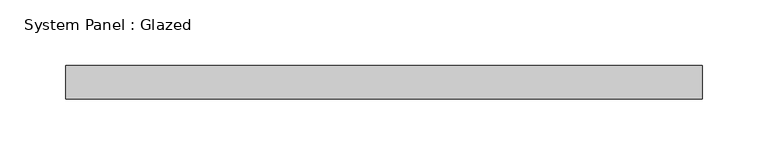
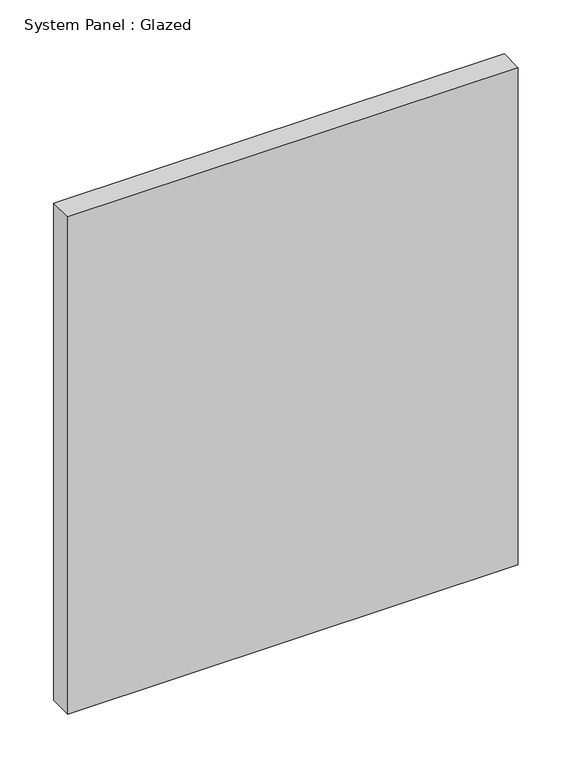
"""IFC4 building model written with IfcOpenShell, lengths in millimetres: plate geometry, System Panel : Glazed."""

from ifc_helpers import new_model, si_unit, origin, origin_with_axes, place, context, project, spatial, polyline, outline, extrude, source, transform, mapped, element, save


def system_panel_glazed_19f1df67(model_context):
    return source(origin(), model_context, "Body", "SweptSolid", [
        extrude(outline(polyline([(241.3, 19.05), (-241.3, 19.05), (-241.3, 44.45), (241.3, 44.45), (241.3, 19.05)])), origin_with_axes(), (0.0, 0.0, 1.0), 562.8451495),
    ])


if __name__ == "__main__":
    model = new_model("IFC4")
    model_context = context("Model", 3, world=origin())
    ifc_project = project(units=[si_unit("LENGTHUNIT", "METRE", prefix="MILLI")], contexts=[model_context])
    site = spatial("IfcSite", under=ifc_project)
    building = spatial("IfcBuilding", under=site)
    placement = place(None, origin())
    system_panel_glazed_shape = system_panel_glazed_19f1df67(model_context)
    element("IfcPlate", 1, ObjectType="System Panel : Glazed", at=placement, inside=building, context=model_context, shape_type="MappedRepresentation", body=[
        mapped(system_panel_glazed_shape, transform((0.0, 0.0, 0.0), x_axis=(1.0, 0.0, 0.0), y_axis=(0.0, 1.0, 0.0), z_axis=(0.0, 0.0, 1.0))),
    ])
    save(model, "model.ifc")

# Revit data of these elements
# Type "System Panel : Glazed"
#   Construction Type Id = "GSP4R"
#   Analytic Construction = "1/8 in Pilkington single glazing"
#   Visual Light Transmittance = 0.9
#   Solar Heat Gain Coefficient = 0.86
#   Heat Transfer Coefficient (U) = 1.18115 BTU/(h·ft²·°F)
#   Define Thermal Properties by = 1
# Element 1 (IfcPlate, "System Panel : Glazed")
#   Materials on its faces: "Glass"
# Materials
#   "Glass": class "Glass", colour RGB 0 128 192, transparency 0.75, Description = "Soda Lime Glass", Cost = 0
